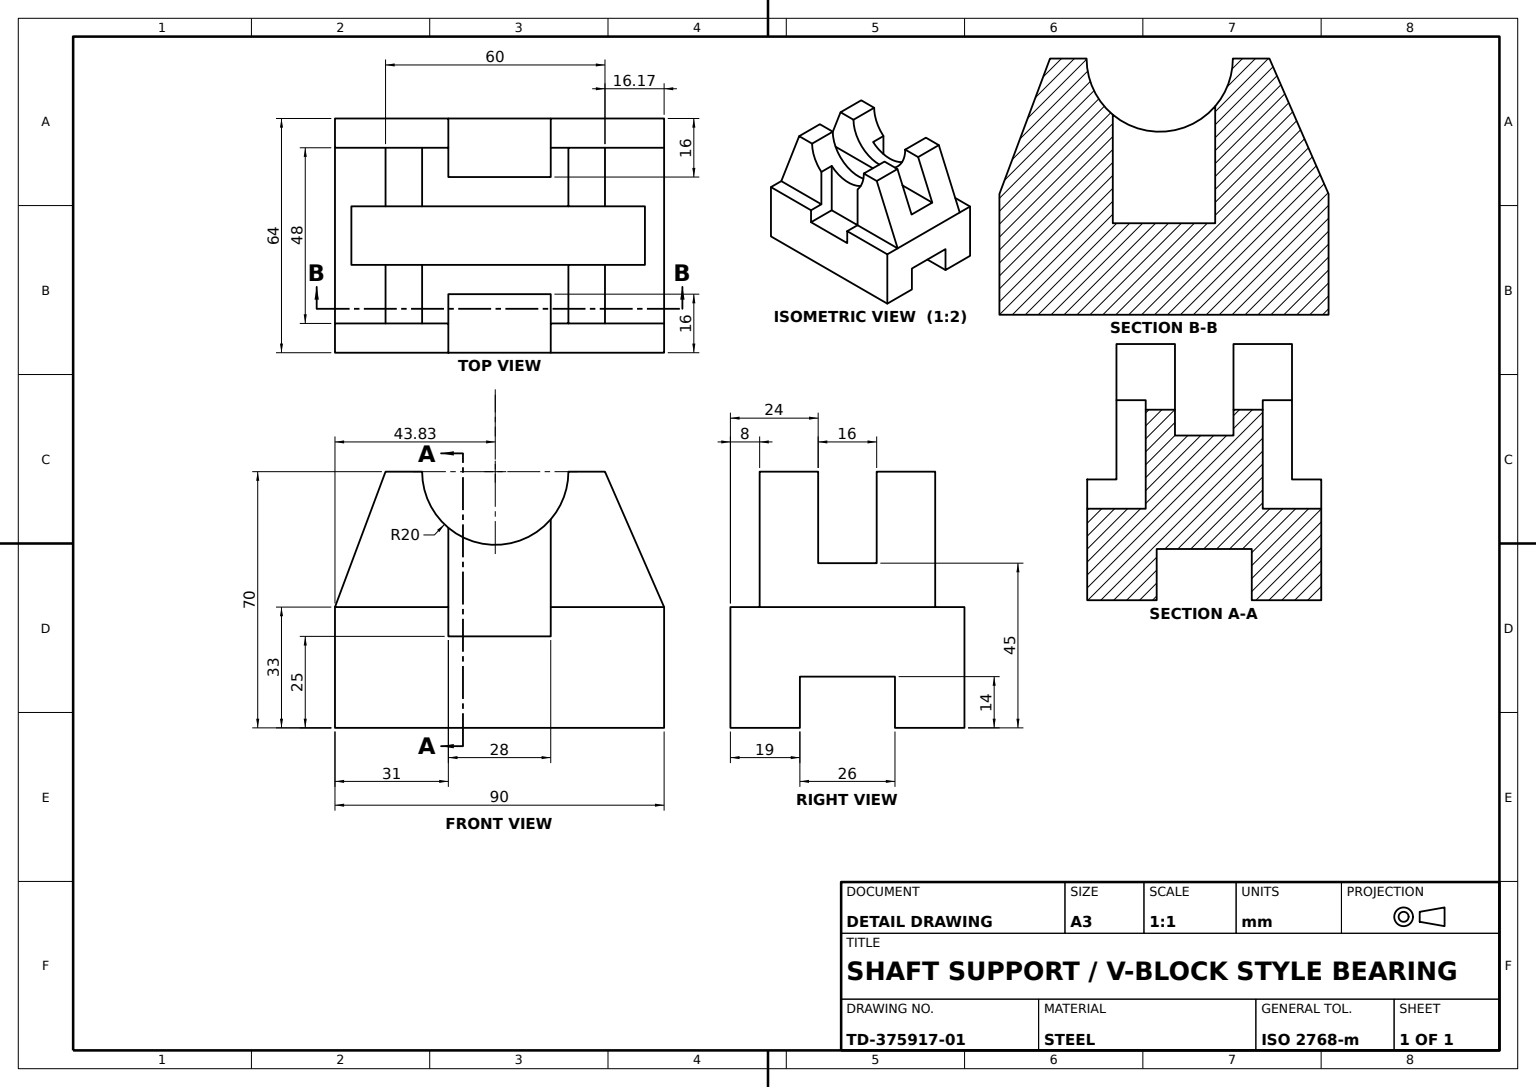
from build123d import *

# Parameters (mm, degrees)
BASE_BLOCK_SKETCH_W     = 90
BASE_BLOCK_SKETCH_H     = 33
BASE_BLOCK_DEPTH        = 32
BOTTOM_SLOT_SKETCH_W    = 26
BOTTOM_SLOT_SKETCH_H    = 14
BOTTOM_SLOT_DEPTH       = 102.05938848
SUPPORT_UPRIGHTS_DEPTH  = 90
CENTRE_RECESS_DEPTH     = 128.027556066
CRADLE_ARC_CUT_DEPTH    = 128.027556066
UPRIGHT_U_SLOT_SKETCH_W = 28
UPRIGHT_U_SLOT_SKETCH_H = 16
UPRIGHT_U_SLOT_DEPTH    = 45


with BuildPart() as part:
    # Base Block Sketch → Base Block (new, symmetric)
    with BuildSketch(Plane.XY):
        with Locations((45, 16.5)):
            Rectangle(BASE_BLOCK_SKETCH_W, BASE_BLOCK_SKETCH_H)
    extrude(amount=BASE_BLOCK_DEPTH, both=True)

    # Bottom Slot Sketch → Bottom Slot (cut, through all)
    with BuildSketch(Plane(origin=(90, 0, 0), x_dir=(0, 0, -1), z_dir=(1, 0, 0))):
        with Locations((0, 7)):
            Rectangle(BOTTOM_SLOT_SKETCH_W, BOTTOM_SLOT_SKETCH_H)
    extrude(amount=-BOTTOM_SLOT_DEPTH, mode=Mode.SUBTRACT)

    # Support Uprights Sketch → Support Uprights (add)
    with BuildSketch(Plane(origin=(90, 0, 0), x_dir=(0, 0, -1), z_dir=(1, 0, 0))):
        Polygon((-24, 33), (24, 33), (24, 70), (8, 70), (8, 45), (-8, 45), (-8, 70), (-24, 70), align=None)
    extrude(amount=-SUPPORT_UPRIGHTS_DEPTH)

    # Centre Recess Sketch → Centre Recess (cut, through all)
    with BuildSketch(Plane.XY.offset(24)):
        Polygon((90, 70), (73.829610801, 70), (90, 33), align=None)
        Polygon((0, 33), (13.829610801, 70), (0, 70), align=None)
    extrude(amount=-CENTRE_RECESS_DEPTH, mode=Mode.SUBTRACT)

    # Cradle Arc Sketch → Cradle Arc Cut (cut, through all)
    with BuildSketch(Plane(origin=(0, 0, -24), x_dir=(-1, 0, 0), z_dir=(0, 0, -1))):
        with BuildLine():
            Line((-23.829610801, 70), (-63.829610801, 70))
            ThreePointArc((-63.829610801, 70), (-43.829610801, 50), (-23.829610801, 70))
        make_face()
    extrude(amount=-CRADLE_ARC_CUT_DEPTH, mode=Mode.SUBTRACT)

    # Upright U-Slot Sketch → Upright U-Slot (cut)
    with BuildSketch(Plane(origin=(0, 70, 0), x_dir=(1, 0, 0), z_dir=(0, 1, 0))):
        with Locations((45, 24)):
            Rectangle(UPRIGHT_U_SLOT_SKETCH_W, UPRIGHT_U_SLOT_SKETCH_H)
        with Locations((45, -24)):
            Rectangle(UPRIGHT_U_SLOT_SKETCH_W, UPRIGHT_U_SLOT_SKETCH_H)
    extrude(amount=-UPRIGHT_U_SLOT_DEPTH, mode=Mode.SUBTRACT)


solid = part.part
